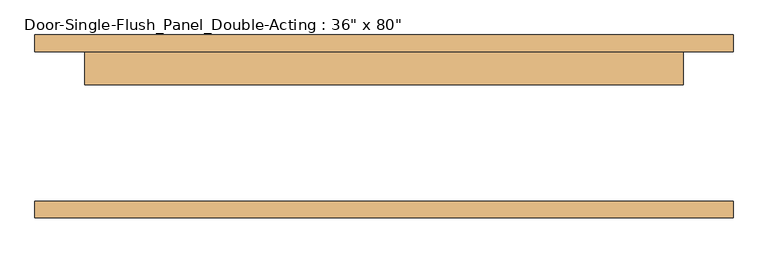
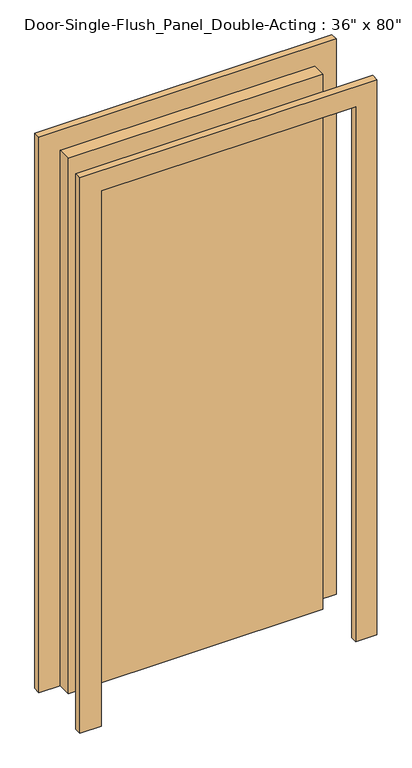
"""IFC4 building model written with IfcOpenShell, lengths in millimetres: door geometry."""

from ifc_helpers import new_model, si_unit, frame, origin, origin_with_axes, place, context, project, spatial, polyline, outline, extrude, source, transform, mapped, element, save


def door_feaa5179(model_context):
    return source(origin(), model_context, "Body", "SweptSolid", [
        extrude(outline(polyline([(457.2, 63.5), (-457.2, 63.5), (-457.2, 114.3), (457.2, 114.3), (457.2, 63.5)])), origin_with_axes(), (0.0, 0.0, 1.0), 2032.0),
        extrude(outline(polyline([(2108.2, 533.4), (2108.2, -533.4), (0.0, -533.4), (0.0, -457.2), (2032.0, -457.2), (2032.0, 457.2), (0.0, 457.2), (0.0, 533.4), (2108.2, 533.4)])), frame((0.0, -139.7, 0.0), z_axis=(0.0, 1.0, 0.0), x_axis=(0.0, 0.0, 1.0)), (0.0, 0.0, 1.0), 25.4),
        extrude(outline(polyline([(2108.2, -533.4), (0.0, -533.4), (0.0, -457.2), (2032.0, -457.2), (2032.0, 457.2), (0.0, 457.2), (0.0, 533.4), (2108.2, 533.4), (2108.2, -533.4)])), frame((0.0, 114.3, 0.0), z_axis=(0.0, 1.0, 0.0), x_axis=(0.0, 0.0, 1.0)), (0.0, 0.0, 1.0), 25.4),
    ])


if __name__ == "__main__":
    model = new_model("IFC4")
    model_context = context("Model", 3, world=origin())
    ifc_project = project(units=[si_unit("LENGTHUNIT", "METRE", prefix="MILLI")], contexts=[model_context])
    site = spatial("IfcSite", under=ifc_project)
    building = spatial("IfcBuilding", under=site)
    placement = place(None, origin())
    door_shape = door_feaa5179(model_context)
    element("IfcDoor", 1, ObjectType="Door-Single-Flush_Panel_Double-Acting : 36\" x 80\"", at=placement, inside=building, context=model_context, shape_type="MappedRepresentation", body=[
        mapped(door_shape, transform((0.0, 0.0, 0.0), x_axis=(1.0, 0.0, 0.0), y_axis=(0.0, 1.0, 0.0), z_axis=(0.0, 0.0, 1.0))),
    ])
    save(model, "model.ifc")

# Revit data of these elements
# Type "Door-Single-Flush_Panel_Double-Acting : 36\" x 80\""
#   Type Mark = "11"
#   Construction Type Id = "DOOR"
#   Assembly Code = "C1020300"
#   Analytic Construction = "Wooden"
#   Thickness = 0' - 2"
#   Thermal Resistance (R) = 2.5876 (h·ft²·°F)/BTU
#   Swing Angle [instance default] = 90.00°
#   Heat Transfer Coefficient (U) = 0.3865 BTU/(h·ft²·°F)
#   Height = 6' - 8"
#   Trim Projection Ext. = 0' - 1"
#   Trim Projection Int. = 0' - 1"
#   Trim Width Ext. = 0' - 3"
#   Trim Width Int. = 0' - 3"
#   Width = 3' - 0"
#   Define Thermal Properties by = 1
#   Trim Material = Paint - Sienna
#   Panel Material = Wood - Birch - Solid Stained Light Low Gloss
#   Visual Light Transmittance = 0
#   Solar Heat Gain Coefficient = 0
#   Function = (empty or 0)
#   Wall Closure = (empty or 0)
# Element 1 (IfcDoor, "Door-Single-Flush_Panel_Double-Acting : 36\" x 80\"")
#   Materials on its faces: "Paint - Sienna", "Wood - Birch - Solid Stained Light Low Gloss"
# Materials
#   "Paint - Sienna": colour RGB 118 70 51, transparency 0, Cost = 0
#   "Wood - Birch - Solid Stained Light Low Gloss": class "Wood", colour RGB 210 159 95, transparency 0, Cost = 0
